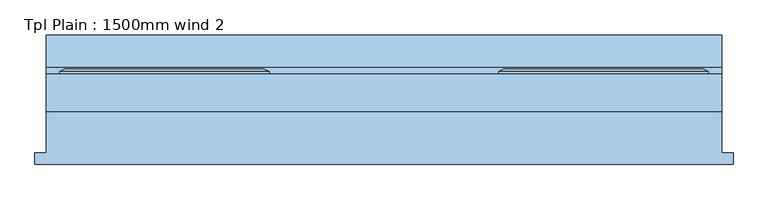
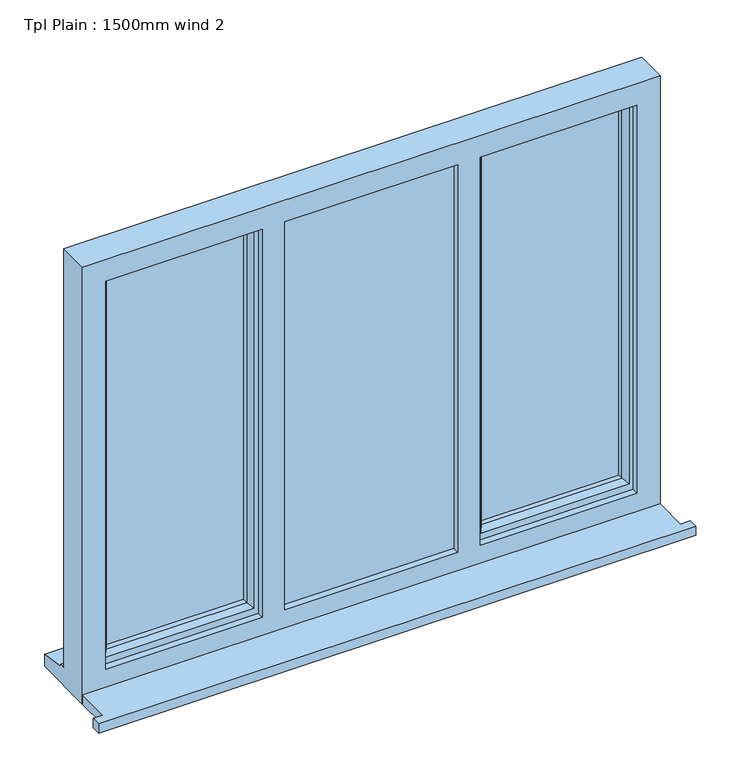
"""IFC4 building model written with IfcOpenShell, lengths in millimetres: window geometry, Tpl Plain : 1500mm wind 2."""

from ifc_helpers import new_model, si_unit, frame, origin, place, context, project, spatial, polyline, outline, extrude, faceted_brep, source, transform, mapped, element, save


def tpl_plain_1500mm_wind_2_30e43110(model_context):
    return source(origin(), model_context, "Body", "SolidModel", [
        extrude(outline(polyline([(-1300.0, -129.0434322), (-1300.0, -104.0434322), (-1275.0, -104.0434322), (-1275.0, -12.0434322), (225.0, -12.0434322), (225.0, -104.0434322), (250.0, -104.0434322), (250.0, -129.0434322), (-1300.0, -129.0434322)])), frame((0.0, 0.0, 1200.0), z_axis=(0.0, 0.0, 1.0), x_axis=(1.0, 0.0, 0.0)), (0.0, 0.0, 1.0), 25.0),
        faceted_brep([(-270.0, 70.9565678, 2370.0), (-270.0, 76.7300705, 2370.0), (-270.0, 76.7300705, 1253.0), (-270.0, 70.9565678, 1253.0), (-260.0, 5.9565678, 2360.0), (-260.0, 70.9565678, 2360.0), (-260.0, 70.9565678, 1263.0), (-260.0, 5.9565678, 1263.0), (-220.0, 20.4494677, 2320.0), (-230.1480377, 5.9565678, 2330.1480377), (-230.1480377, 5.9565678, 1292.8519623), (-220.0, 20.4494677, 1303.0), (-220.0, 34.9565678, 2320.0), (-220.0, 34.9565678, 1303.0), (-230.0, 58.9565678, 2330.0), (-230.0, 34.9565678, 2330.0), (-230.0, 34.9565678, 1293.0), (-230.0, 58.9565678, 1293.0), (-220.0, 76.7300705, 2320.0), (-220.0, 58.9565678, 2320.0), (-220.0, 58.9565678, 1303.0), (-220.0, 76.7300705, 1303.0), (-237.4457548, 82.5035732, 2337.4457548), (-237.4457548, 82.5035732, 1285.5542452), (-259.2153903, 82.5035732, 2359.2153903), (-259.2153903, 82.5035732, 1263.7846097), (195.0, 76.7300705, 1253.0), (195.0, 70.9565678, 1253.0), (185.0, 70.9565678, 1263.0), (185.0, 5.9565678, 1263.0), (155.1480377, 5.9565678, 1292.8519623), (145.0, 20.4494677, 1303.0), (145.0, 34.9565678, 1303.0), (155.0, 34.9565678, 1293.0), (155.0, 58.9565678, 1293.0), (145.0, 58.9565678, 1303.0), (145.0, 76.7300705, 1303.0), (162.4457548, 82.5035732, 1285.5542452), (184.2153903, 82.5035732, 1263.7846097), (195.0, 76.7300705, 2370.0), (195.0, 70.9565678, 2370.0), (185.0, 70.9565678, 2360.0), (185.0, 5.9565678, 2360.0), (155.1480377, 5.9565678, 2330.1480377), (145.0, 20.4494677, 2320.0), (145.0, 34.9565678, 2320.0), (155.0, 34.9565678, 2330.0), (155.0, 58.9565678, 2330.0), (145.0, 58.9565678, 2320.0), (145.0, 76.7300705, 2320.0), (162.4457548, 82.5035732, 2337.4457548), (184.2153903, 82.5035732, 2359.2153903)], [[[0, 1, 2, 3]], [[4, 5, 6, 7]], [[8, 9, 10, 11]], [[12, 8, 11, 13]], [[14, 15, 16, 17]], [[18, 19, 20, 21]], [[22, 18, 21, 23]], [[1, 24, 25, 2]], [[3, 2, 26, 27]], [[7, 6, 28, 29]], [[11, 10, 30, 31]], [[13, 11, 31, 32]], [[17, 16, 33, 34]], [[21, 20, 35, 36]], [[23, 21, 36, 37]], [[2, 25, 38, 26]], [[27, 26, 39, 40]], [[29, 28, 41, 42]], [[31, 30, 43, 44]], [[32, 31, 44, 45]], [[34, 33, 46, 47]], [[36, 35, 48, 49]], [[37, 36, 49, 50]], [[26, 38, 51, 39]], [[40, 39, 1, 0]], [[3, 27, 40, 0], [5, 41, 28, 6]], [[42, 41, 5, 4]], [[7, 29, 42, 4], [9, 43, 30, 10]], [[44, 43, 9, 8]], [[45, 44, 8, 12]], [[15, 46, 33, 16], [13, 32, 45, 12]], [[47, 46, 15, 14]], [[17, 34, 47, 14], [19, 48, 35, 20]], [[49, 48, 19, 18]], [[50, 49, 18, 22]], [[24, 51, 38, 25], [23, 37, 50, 22]], [[39, 51, 24, 1]]]),
        faceted_brep([(-780.0, 70.9565678, 2370.0), (-780.0, 76.7300705, 2370.0), (-1245.0, 76.7300705, 2370.0), (-1245.0, 70.9565678, 2370.0), (-790.0, 5.9565678, 2360.0), (-790.0, 70.9565678, 2360.0), (-1235.0, 70.9565678, 2360.0), (-1235.0, 5.9565678, 2360.0), (-830.0, 20.4494677, 2320.0), (-819.8519623, 5.9565678, 2330.1480377), (-1205.1480377, 5.9565678, 2330.1480377), (-1195.0, 20.4494677, 2320.0), (-830.0, 34.9565678, 2320.0), (-1195.0, 34.9565678, 2320.0), (-820.0, 58.9565678, 2330.0), (-820.0, 34.9565678, 2330.0), (-1205.0, 34.9565678, 2330.0), (-1205.0, 58.9565678, 2330.0), (-830.0, 76.7300705, 2320.0), (-830.0, 58.9565678, 2320.0), (-1195.0, 58.9565678, 2320.0), (-1195.0, 76.7300705, 2320.0), (-811.1854344, 82.5035732, 2338.8145656), (-1213.8145656, 82.5035732, 2338.8145656), (-791.6307806, 82.5035732, 2358.3692194), (-1233.3692194, 82.5035732, 2358.3692194), (-1245.0, 76.7300705, 1253.0), (-1245.0, 70.9565678, 1253.0), (-1235.0, 70.9565678, 1263.0), (-1235.0, 5.9565678, 1263.0), (-1205.1480377, 5.9565678, 1292.8519623), (-1195.0, 20.4494677, 1303.0), (-1195.0, 34.9565678, 1303.0), (-1205.0, 34.9565678, 1293.0), (-1205.0, 58.9565678, 1293.0), (-1195.0, 58.9565678, 1303.0), (-1195.0, 76.7300705, 1303.0), (-1213.8145656, 82.5035732, 1284.1854344), (-1233.3692194, 82.5035732, 1264.6307806), (-780.0, 76.7300705, 1253.0), (-780.0, 70.9565678, 1253.0), (-790.0, 70.9565678, 1263.0), (-790.0, 5.9565678, 1263.0), (-819.8519623, 5.9565678, 1292.8519623), (-830.0, 20.4494677, 1303.0), (-830.0, 34.9565678, 1303.0), (-820.0, 34.9565678, 1293.0), (-820.0, 58.9565678, 1293.0), (-830.0, 58.9565678, 1303.0), (-830.0, 76.7300705, 1303.0), (-811.1854344, 82.5035732, 1284.1854344), (-791.6307806, 82.5035732, 1264.6307806)], [[[0, 1, 2, 3]], [[4, 5, 6, 7]], [[8, 9, 10, 11]], [[12, 8, 11, 13]], [[14, 15, 16, 17]], [[18, 19, 20, 21]], [[22, 18, 21, 23]], [[1, 24, 25, 2]], [[3, 2, 26, 27]], [[7, 6, 28, 29]], [[11, 10, 30, 31]], [[13, 11, 31, 32]], [[17, 16, 33, 34]], [[21, 20, 35, 36]], [[23, 21, 36, 37]], [[2, 25, 38, 26]], [[27, 26, 39, 40]], [[0, 3, 27, 40], [41, 28, 6, 5]], [[29, 28, 41, 42]], [[4, 7, 29, 42], [43, 30, 10, 9]], [[31, 30, 43, 44]], [[32, 31, 44, 45]], [[46, 33, 16, 15], [12, 13, 32, 45]], [[34, 33, 46, 47]], [[14, 17, 34, 47], [48, 35, 20, 19]], [[36, 35, 48, 49]], [[37, 36, 49, 50]], [[51, 38, 25, 24], [22, 23, 37, 50]], [[26, 38, 51, 39]], [[40, 39, 1, 0]], [[42, 41, 5, 4]], [[44, 43, 9, 8]], [[45, 44, 8, 12]], [[47, 46, 15, 14]], [[49, 48, 19, 18]], [[50, 49, 18, 22]], [[39, 51, 24, 1]]]),
        faceted_brep([(225.0, -12.0434322, 2400.0), (-1275.0, -12.0434322, 2400.0), (-1275.0, -12.0434322, 1200.0), (225.0, -12.0434322, 1200.0), (165.0, -12.0434322, 2340.0), (165.0, -12.0434322, 1275.0), (-242.0, -12.0434322, 1275.0), (-242.0, -12.0434322, 2340.0), (-300.0, -12.0434322, 2340.0), (-300.0, -12.0434322, 1275.0), (-750.0, -12.0434322, 1275.0), (-750.0, -12.0434322, 2340.0), (-808.0, -12.0434322, 2340.0), (-808.0, -12.0434322, 1275.0), (-1215.0, -12.0434322, 1275.0), (-1215.0, -12.0434322, 2340.0), (-1275.0, 70.9565678, 2400.0), (-1275.0, 70.9565678, 1251.0), (-1275.0, 85.9565678, 1249.68767), (-1275.0, 85.9565678, 1244.7449676), (-1275.0, 158.4565678, 1233.8088847), (-1275.0, 158.4565678, 1200.0), (225.0, 70.9565678, 2400.0), (225.0, 70.9565678, 1251.0), (-1235.0, 70.9565678, 2360.0), (-1235.0, 70.9565678, 1263.0), (-790.0, 70.9565678, 1263.0), (-790.0, 70.9565678, 2360.0), (-750.0, 70.9565678, 2360.0), (-750.0, 70.9565678, 1263.0), (-300.0, 70.9565678, 1263.0), (-300.0, 70.9565678, 2360.0), (-260.0, 70.9565678, 2360.0), (-260.0, 70.9565678, 1263.0), (185.0, 70.9565678, 1263.0), (185.0, 70.9565678, 2360.0), (-1235.0, 5.9565678, 2360.0), (-1235.0, 5.9565678, 1263.0), (-760.0, 5.9565678, 2360.0), (-290.0, 5.9565678, 2360.0), (-290.0, 5.9565678, 1263.0), (-760.0, 5.9565678, 1263.0), (-300.0, 5.9565678, 2340.0), (-750.0, 5.9565678, 2340.0), (-750.0, 5.9565678, 1275.0), (-300.0, 5.9565678, 1275.0), (-260.0, 5.9565678, 2360.0), (185.0, 5.9565678, 2360.0), (185.0, 5.9565678, 1263.0), (-260.0, 5.9565678, 1263.0), (165.0, 5.9565678, 2340.0), (-242.0, 5.9565678, 2340.0), (-242.0, 5.9565678, 1275.0), (165.0, 5.9565678, 1275.0), (-790.0, 5.9565678, 2360.0), (-790.0, 5.9565678, 1263.0), (-808.0, 5.9565678, 2340.0), (-1215.0, 5.9565678, 2340.0), (-1215.0, 5.9565678, 1275.0), (-808.0, 5.9565678, 1275.0), (-750.0, 29.9565678, 2360.0), (-300.0, 29.9565678, 2360.0), (-290.0, 29.9565678, 2360.0), (-760.0, 29.9565678, 2360.0), (225.0, 158.4565678, 1200.0), (225.0, 158.4565678, 1233.8088847), (225.0, 85.9565678, 1244.7449676), (225.0, 85.9565678, 1249.68767), (-750.0, 29.9565678, 1263.0), (-760.0, 29.9565678, 1263.0), (-290.0, 29.9565678, 1263.0), (-300.0, 29.9565678, 1263.0)], [[[0, 1, 2, 3], [4, 5, 6, 7], [8, 9, 10, 11], [12, 13, 14, 15]], [[2, 1, 16, 17, 18, 19, 20, 21]], [[17, 16, 22, 23], [24, 25, 26, 27], [28, 29, 30, 31], [32, 33, 34, 35]], [[25, 24, 36, 37]], [[38, 39, 40, 41], [42, 43, 44, 45]], [[46, 47, 48, 49], [50, 51, 52, 53]], [[36, 54, 55, 37], [56, 57, 58, 59]], [[57, 15, 14, 58]], [[1, 0, 22, 16]], [[36, 24, 27, 54]], [[35, 47, 46, 32]], [[60, 28, 31, 61, 62, 39, 38, 63]], [[15, 57, 56, 12]], [[50, 4, 7, 51]], [[11, 43, 42, 8]], [[23, 22, 0, 3, 64, 65, 66, 67]], [[35, 34, 48, 47]], [[4, 50, 53, 5]], [[43, 11, 10, 44]], [[12, 56, 59, 13]], [[27, 26, 55, 54]], [[29, 28, 60, 68]], [[68, 60, 63, 69]], [[69, 63, 38, 41]], [[62, 70, 40, 39]], [[70, 62, 61, 71]], [[71, 61, 31, 30]], [[33, 32, 46, 49]], [[51, 7, 6, 52]], [[8, 42, 45, 9]], [[64, 3, 2, 21]], [[65, 64, 21, 20]], [[66, 65, 20, 19]], [[67, 66, 19, 18]], [[23, 67, 18, 17]], [[26, 25, 37, 55]], [[34, 33, 49, 48]], [[41, 40, 70, 71, 30, 29, 68, 69]], [[6, 5, 53, 52]], [[45, 44, 10, 9]], [[59, 58, 14, 13]]]),
        extrude(outline(polyline([(-820.0, 34.9565678), (-1205.0, 34.9565678), (-1205.0, 58.9565678), (-820.0, 58.9565678), (-820.0, 34.9565678)])), frame((0.0, 0.0, 1293.0), z_axis=(0.0, 0.0, 1.0), x_axis=(1.0, 0.0, 0.0)), (0.0, 0.0, 1.0), 1037.0),
        extrude(outline(polyline([(-760.0, 29.9565678), (-290.0, 29.9565678), (-290.0, 5.9565678), (-760.0, 5.9565678), (-760.0, 29.9565678)])), frame((0.0, 0.0, 1263.0), z_axis=(0.0, 0.0, 1.0), x_axis=(1.0, 0.0, 0.0)), (0.0, 0.0, 1.0), 1097.0),
        extrude(outline(polyline([(155.0, 34.9565678), (-230.0, 34.9565678), (-230.0, 58.9565678), (155.0, 58.9565678), (155.0, 34.9565678)])), frame((0.0, 0.0, 1293.0), z_axis=(0.0, 0.0, 1.0), x_axis=(1.0, 0.0, 0.0)), (0.0, 0.0, 1.0), 1037.0),
    ])


if __name__ == "__main__":
    model = new_model("IFC4")
    model_context = context("Model", 3, world=origin())
    ifc_project = project(units=[si_unit("LENGTHUNIT", "METRE", prefix="MILLI")], contexts=[model_context])
    site = spatial("IfcSite", under=ifc_project)
    building = spatial("IfcBuilding", under=site)
    placement = place(None, origin())
    tpl_plain_1500mm_wind_2_shape = tpl_plain_1500mm_wind_2_30e43110(model_context)
    element("IfcWindow", 1, ObjectType="Tpl Plain : 1500mm wind 2", at=placement, inside=building, context=model_context, shape_type="MappedRepresentation", body=[
        mapped(tpl_plain_1500mm_wind_2_shape, transform((0.0, 0.0, 0.0), x_axis=(1.0, 0.0, 0.0), y_axis=(0.0, 1.0, 0.0), z_axis=(0.0, 0.0, 1.0))),
    ])
    save(model, "model.ifc")

# Revit data of these elements
# Type "Tpl Plain : 1500mm wind 2"
#   Type Mark = "37"
#   Operation = "TriplePanelVertical"
#   Manufacturer = "Revit"
#   Keynote = "L10"
#   Analytic Construction = "<None>"
#   Wrap Layers (Ext) from Ext = 102.5 mm
#   Wrap Layers (Int) from Ext = 177.5 mm
#   Window Board Projection = 25 mm
#   Window Board Extension = 25 mm
#   Rough Width = 1500 mm
#   Rough Height = 1200 mm
#   Height = 1200 mm
#   Width = 1500 mm
#   Glazing Thickness = 24 mm
#   FrameOffset - External = 50 mm
#   Frame Depth = 65 mm
#   Default Head Height = 2400 mm
#   Cill Depth = 87.5 mm
#   Cavity Closer Width = 50 mm
#   Cavity Closer Offset from Ext = 102.5 mm
#   Cavity Closer Depth = 85 mm
#   Vis - Cavity Closers = yes
#   Define Thermal Properties by = 1
#   Material Trim = Window Frame
#   Material Glass = Glass
#   Material Frame = Window Frame
#   Wall Closure = (empty or 0)
# Element 1 (IfcWindow, "Tpl Plain : 1500mm wind 2")
#   Materials on its faces: "Window Frame", "Glass"
# Materials
#   "Window Frame": colour RGB 249 249 249, transparency 0, Keynote = "L10", Cost = 0
#   "Glass": class "Glass", colour RGB 0 128 192, transparency 0.9, Description = "Soda Lime Glass", Cost = 0
